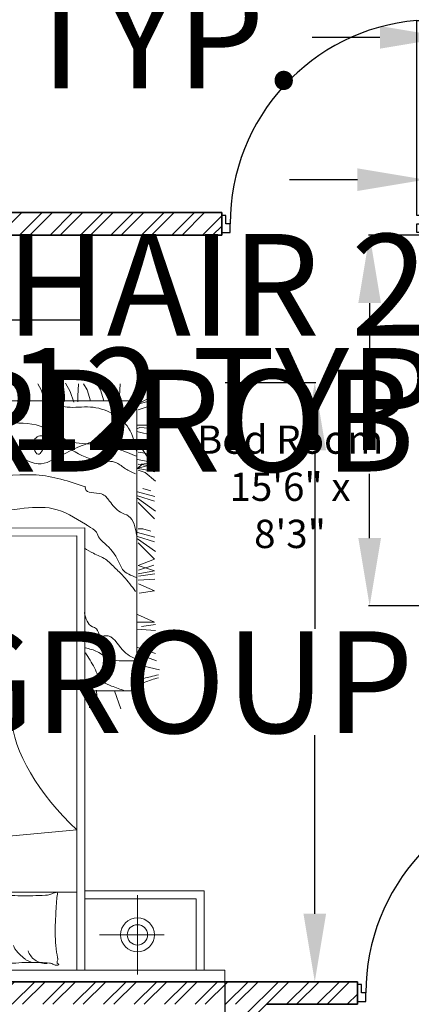
# Model space of a CAD drawing. Units: inches. Extents: x -90 to 536, y -553 to 299.
# Tile 20 of 27: x 137 to 207, y -2 to 173. Entities that reach past the tile are written whole.
import ezdxf

# ---------------------------------------------------------------- set-up
doc = ezdxf.new("R2010")
doc.units = ezdxf.units.IN
for name, color, linetype, lineweight in [('A-ANNO-DIMS', 2, 'Continuous', 18), ('A-AREA-IDEN', 7, 'Continuous', 18), ('A-DOOR', 4, 'Continuous', 25), ('A-FLOR-CASE', 2, 'Continuous', 25), ('A-WALL-PATT', 252, 'Continuous', 13), ('Furniture', 2, 'Continuous', 18), ('Inner Wall', 5, 'Continuous', 35)]:
    doc.layers.add(name, color=color, linetype=linetype, lineweight=lineweight)
doc.styles.get("Standard").update_dxf_attribs({"font": 'arial.ttf'})
doc.dimstyles.get("Standard").update_dxf_attribs({"dimtxt": 18, "dimasz": 12, "dimexe": 0.18, "dimexo": 0.0625, "dimgap": 0.09, "dimtad": 0, "dimtih": 1, "dimtoh": 1, "dimdec": 0, "dimzin": 0, "dimdsep": 46, "dimlunit": 3, "dimtxsty": 'Standard', "dimcen": 0.09, "dimadec": 0, "dimazin": 0, "dimtfac": 1, "dimtdec": 0, "dimtofl": 0, "dimtmove": 0, "dimatfit": 3, "dimfxl": 1, "dimtolj": 1, "dimtzin": 0, "dimarcsym": 0})

# ---------------------------------------------------------------- blocks, each defined once
blk = doc.blocks.new('A$C2B723114')
for p, q in [((0, 2.9047), (2.8274, 2.9047)), ((0, 2.8487), (0, 2.9047)), ((0.4243, 2.8697), (0.4243, 2.4855)), ((2.4742, 2.8697), (2.4742, 2.4855)), ((2.8274, 2.9047), (2.8274, 2.8487)), ((2.8274, 2.8487), (0, 2.8487)), ((0.1012, 2.4649), (0.1012, 2.849)), ((0.1396, 2.5033), (0.1396, 2.849)), ((0.6794, 0.7051), (0.6794, 2.8509)), ((0.7187, 0.7435), (0.7187, 2.8509)), ((2.1776, 2.8509), (2.1776, 0.7454)), ((2.216, 2.8509), (2.216, 0.707)), ((2.6798, 2.5052), (2.6798, 2.8509)), ((2.7182, 2.4668), (2.7182, 2.8509)), ((0.6087, 2.6776), (0.295, 2.6776)), ((2.6586, 2.6776), (2.2821, 2.6776)), ((1.3789, 2.4999), (1.3598, 2.5761)), ((2.0593, 2.4999), (2.0402, 2.5761)), ((0.6766, 2.5033), (0.1396, 2.5033)), ((1.3858, 2.4723), (1.3789, 2.4999)), ((2.0662, 2.4723), (2.0593, 2.4999)), ((2.2188, 2.5052), (2.6798, 2.5052)), ((0.6794, 2.4649), (0.1012, 2.4649)), ((0.7191, 2.47), (2.1778, 2.4719)), ((2.2188, 2.4668), (2.7182, 2.4668)), ((2.1771, 2.3036), (0.718, 2.1685)), ((1.0365, 1.6233), (2.1246, 2.2989)), ((0.5047, 1.5819), (0.5353, 1.4945)), ((0.6174, 1.5819), (0.6232, 1.4916)), ((0.6467, 1.5819), (0.6369, 1.5137)), ((0.6571, 1.4945), (0.6571, 1.5765)), ((2.2287, 1.6076), (2.2523, 1.5035)), ((2.2726, 1.593), (2.3061, 1.5007)), ((2.3067, 1.5881), (2.3373, 1.5007)), ((2.4194, 1.5881), (2.4251, 1.4979)), ((2.4487, 1.5881), (2.4389, 1.5199)), ((2.4591, 1.5007), (2.4591, 1.5828)), ((0.4269, 0.0884), (0.4269, 1.4945)), ((0.4269, 1.4945), (0.6794, 1.4945)), ((2.4685, 1.4964), (2.216, 1.5022)), ((2.4685, 1.4964), (2.4685, 0.0903)), ((0.3172, 1.3923), (0.4213, 1.3687)), ((2.4685, 1.4044), (2.5491, 1.3861)), ((0.3318, 1.3485), (0.4241, 1.3149)), ((2.4596, 1.3659), (2.552, 1.3324)), ((0.3367, 1.3143), (0.4241, 1.2838)), ((2.4645, 1.3318), (2.552, 1.3012)), ((2.4645, 1.2928), (2.5548, 1.2871)), ((2.4645, 1.2635), (2.5328, 1.2733)), ((2.4699, 1.2531), (2.552, 1.2163)), ((2.552, 1.2531), (2.4699, 1.2531)), ((0.3367, 1.2016), (0.427, 1.1959)), ((2.5435, 1.2276), (2.4699, 1.2163)), ((2.4699, 1.2163), (2.5463, 1.1823)), ((0.3367, 1.1724), (0.405, 1.1821)), ((0.4241, 1.162), (0.3421, 1.162)), ((0.3421, 1.162), (0.4241, 1.1252)), ((2.5491, 1.1654), (2.467, 1.1597)), ((2.5463, 1.1455), (2.467, 1.1342)), ((2.5491, 1.1342), (2.4699, 1.1201)), ((2.4699, 1.1201), (2.5491, 1.0946)), ((2.5463, 1.1172), (2.4727, 1.0918)), ((2.5491, 1.0946), (2.4699, 1.0635)), ((2.4699, 1.0635), (2.5491, 0.9842)), ((0.4157, 1.0206), (0.3421, 1.0093)), ((0.3421, 1.0093), (0.4185, 0.9754)), ((2.4642, 1.0267), (2.552, 0.9644)), ((0.4213, 0.9584), (0.3392, 0.9527)), ((2.467, 0.9559), (2.552, 0.9333)), ((2.4699, 0.9785), (2.552, 0.9531)), ((0.4185, 0.9386), (0.3392, 0.9272)), ((0.4213, 0.9272), (0.3421, 0.9131)), ((0.3421, 0.9131), (0.4213, 0.8876)), ((0.4185, 0.9103), (0.3449, 0.8848)), ((2.4642, 0.9389), (2.4869, 0.9276)), ((2.4869, 0.9276), (2.5265, 0.9163)), ((2.5265, 0.9163), (2.5491, 0.9163)), ((0.4213, 0.8876), (0.3421, 0.8565)), ((2.4642, 0.8908), (2.5152, 0.8483)), ((0.3364, 0.8197), (0.4241, 0.7574)), ((0.3421, 0.8565), (0.4213, 0.7772)), ((2.467, 0.8455), (2.5208, 0.8342)), ((2.4699, 0.8172), (2.4925, 0.7974)), ((2.5491, 0.8087), (2.4699, 0.8172)), ((2.5152, 0.8483), (2.5491, 0.837)), ((2.5208, 0.8342), (2.552, 0.8285)), ((2.552, 0.8285), (2.5293, 0.8087)), ((0.3421, 0.7716), (0.4241, 0.7461)), ((2.5491, 0.7606), (2.467, 0.7719)), ((2.4925, 0.7974), (2.535, 0.7889)), ((2.535, 0.7889), (2.552, 0.7861)), ((0.3392, 0.7489), (0.4241, 0.7263)), ((0.359, 0.7206), (0.3987, 0.7093)), ((2.1776, 0.7454), (0.7187, 0.7435)), ((2.4727, 0.7464), (2.467, 0.7408)), ((2.467, 0.7153), (2.5491, 0.7238)), ((2.552, 0.7464), (2.4727, 0.7464)), ((0.3987, 0.7093), (0.4213, 0.7093)), ((2.216, 0.707), (0.6794, 0.7051)), ((0.9938, 0.6115), (1.7555, 0.7064)), ((2.5491, 0.6842), (2.4642, 0.6615)), ((2.552, 0.7096), (2.467, 0.6842)), ((0.3364, 0.6233), (0.4241, 0.561)), ((0.3421, 0.6601), (0.4213, 0.5808)), ((2.5491, 0.6672), (2.4755, 0.6587)), ((2.4755, 0.6474), (2.5548, 0.6276)), ((0.3421, 0.5752), (0.4241, 0.5497)), ((2.4642, 0.6191), (2.4784, 0.6134)), ((2.467, 0.5993), (2.4869, 0.5964)), ((2.4784, 0.6134), (2.5406, 0.6077)), ((2.4869, 0.5964), (2.552, 0.5964)), ((2.5406, 0.6077), (2.552, 0.6134)), ((0.3392, 0.5525), (0.4241, 0.5299)), ((2.467, 0.5313), (2.5491, 0.5596)), ((2.467, 0.5087), (2.5548, 0.5342)), ((2.5548, 0.5342), (2.4699, 0.4889)), ((0.3364, 0.4785), (0.3874, 0.436)), ((0.359, 0.5242), (0.3987, 0.5129)), ((1.4523, 0.5021), (1.1305, 0.4537)), ((0.3392, 0.4332), (0.393, 0.4219)), ((0.3874, 0.436), (0.4213, 0.4247)), ((1.1305, 0.4537), (0.9938, 0.448)), ((0.4213, 0.415), (0.3364, 0.3923)), ((0.4241, 0.2868), (0.3392, 0.415)), ((0.3421, 0.4049), (0.3647, 0.3851)), ((0.4213, 0.3964), (0.3421, 0.4049)), ((0.4213, 0.398), (0.3477, 0.3895)), ((0.3647, 0.3851), (0.4072, 0.3766)), ((0.393, 0.4219), (0.4241, 0.4162)), ((0.4241, 0.4162), (0.4015, 0.3964)), ((2.467, 0.4133), (2.552, 0.4019)), ((2.467, 0.2879), (2.552, 0.4076)), ((0.4213, 0.3377), (0.3392, 0.3491)), ((0.4072, 0.3766), (0.4241, 0.3738)), ((0.3392, 0.2925), (0.4213, 0.3009)), ((0.4241, 0.3236), (0.3449, 0.3236)), ((2.4642, 0.3049), (2.5491, 0.2851)), ((2.467, 0.319), (2.5548, 0.3134)), ((0.3477, 0.2571), (0.427, 0.2373)), ((2.4699, 0.2491), (2.501, 0.2491)), ((2.501, 0.2491), (2.5491, 0.2547)), ((0.3506, 0.2231), (0.4128, 0.2175)), ((0.359, 0.2061), (0.4241, 0.2061)), ((0.4128, 0.2175), (0.4241, 0.2231)), ((2.467, 0.2179), (2.5605, 0.1981)), ((2.467, 0.1981), (2.5491, 0.1613)), ((2.467, 0.184), (2.4982, 0.1755)), ((2.4982, 0.1755), (2.5463, 0.1359)), ((0.3392, 0.1042), (0.4213, 0.1325)), ((0.3392, 0.0815), (0.427, 0.107)), ((0.427, 0.107), (0.3421, 0.0617)), ((1.5674, 0.0962), (1.5844, 0.0453)), ((1.8568, 0.0962), (1.8738, 0.0453)), ((1.9342, 0.0962), (1.9512, 0.0453)), ((2.2236, 0.0962), (2.2406, 0.0453)), ((2.4642, 0.0991), (2.5378, 0.0877)), ((2.4699, 0.1302), (2.535, 0.1104)), ((2.535, 0.1104), (2.5491, 0.0991)), ((2.4685, 0.0903), (0.4269, 0.0884)), ((0.5106, 0.0657), (0.5077, 0.0063)), ((0.5106, 0.094), (0.5106, 0.0657)), ((0.5417, 0.094), (0.5474, 0.0572)), ((0.5474, 0.0572), (0.57, 0.0006)), ((0.587, 0.0884), (0.604, 0.0346)), ((0.6512, 0.0884), (0.6682, 0.0346)), ((0.713, 0.0657), (0.7101, 0.0063)), ((0.713, 0.094), (0.713, 0.0657)), ((0.7334, 0.0943), (0.7503, 0.0434)), ((0.7786, 0.0915), (0.7786, 0.0632)), ((0.7786, 0.0632), (0.7843, 0.0066)), ((0.8739, 0.0884), (0.8908, 0.0346)), ((0.956, 0.0943), (0.973, 0.0434)), ((1.0013, 0.0915), (1.0013, 0.0632)), ((1.0013, 0.0632), (1.007, 0.0066)), ((1.072, 0.0884), (1.089, 0.0346)), ((1.1338, 0.0657), (1.131, 0.0063)), ((1.1338, 0.094), (1.1338, 0.0657)), ((1.1542, 0.0943), (1.1712, 0.0434)), ((1.1995, 0.0915), (1.1995, 0.0632)), ((1.1995, 0.0632), (1.2052, 0.0066)), ((1.4088, 0.0657), (1.406, 0.0063)), ((1.4088, 0.094), (1.4088, 0.0657)), ((1.44, 0.094), (1.4456, 0.0572)), ((1.4456, 0.0572), (1.4683, 0.0006)), ((1.4853, 0.0884), (1.5023, 0.0346)), ((1.6127, 0.0934), (1.6127, 0.0651)), ((1.6127, 0.0651), (1.6184, 0.0085)), ((1.6297, 0.0849), (1.624, 0.0028)), ((1.6693, 0.0623), (1.6608, 0.0028)), ((1.6721, 0.0877), (1.6693, 0.0623)), ((1.7344, 0.0651), (1.7316, 0.0057)), ((1.7344, 0.0934), (1.7344, 0.0651)), ((1.7655, 0.0934), (1.7712, 0.0566)), ((1.7712, 0.0566), (1.7938, 0)), ((1.8108, 0.0877), (1.8278, 0.034)), ((1.9795, 0.0934), (1.9795, 0.0651)), ((1.9795, 0.0651), (1.9852, 0.0085)), ((1.9965, 0.0849), (1.9908, 0.0028)), ((2.0361, 0.0623), (2.0276, 0.0028)), ((2.039, 0.0877), (2.0361, 0.0623)), ((2.1012, 0.0651), (2.0984, 0.0057)), ((2.1012, 0.0934), (2.1012, 0.0651)), ((2.1324, 0.0934), (2.138, 0.0566)), ((2.138, 0.0566), (2.1607, 0)), ((2.1777, 0.0877), (2.1946, 0.034)), ((2.2689, 0.0934), (2.2689, 0.0651)), ((2.2689, 0.0651), (2.2746, 0.0085)), ((2.2859, 0.0849), (2.2802, 0.0028)), ((2.3255, 0.0623), (2.317, 0.0028)), ((2.3284, 0.0877), (2.3255, 0.0623)), ((2.3906, 0.0651), (2.3878, 0.0057)), ((2.3906, 0.0934), (2.3906, 0.0651)), ((2.4218, 0.0934), (2.4274, 0.0566)), ((2.4274, 0.0566), (2.4501, 0)), ((2.467, 0.0877), (2.484, 0.034)), ((2.5378, 0.0877), (2.5463, 0.0821)), ((0.604, 0.0346), (0.621, 0.0063)), ((0.6682, 0.0346), (0.6851, 0.0063)), ((0.7503, 0.0434), (0.773, 0.0037)), ((0.8908, 0.0346), (0.9078, 0.0063)), ((0.973, 0.0434), (0.9957, 0.0037)), ((1.089, 0.0346), (1.106, 0.0063)), ((1.1712, 0.0434), (1.1939, 0.0037)), ((1.5023, 0.0346), (1.5192, 0.0082)), ((1.5844, 0.0453), (1.607, 0.0057)), ((1.8278, 0.034), (1.8448, 0.0057)), ((1.8738, 0.0453), (1.8964, 0.0057)), ((1.9512, 0.0453), (1.9739, 0.0057)), ((2.1946, 0.034), (2.2116, 0.0057)), ((2.2406, 0.0453), (2.2632, 0.0057)), ((2.484, 0.034), (2.501, 0.0057))]:
    blk.add_line(p, q)
for centre, radius in [((0.4243, 2.6776), 0.0821), ((0.4243, 2.6776), 0.0493), ((2.4742, 2.6776), 0.0821), ((2.4742, 2.6776), 0.0493)]:
    blk.add_circle(centre, radius)
for centre, radius, start, end in [((0.8078, 2.821), 0.00214, 160.436, 281.8931), ((0.8088, 2.8207), 0.00315, 111.7883, 160.436), ((0.8162, 2.8021), 0.0232, 94.3025, 111.7883), ((0.8091, 2.8151), 0.00394, 21.9904, 101.8931), ((0.7994, 2.8112), 0.0144, 338.579, 21.9904), ((0.8165, 2.7987), 0.0266, 59.3487, 94.3025), ((0.8554, 2.8643), 0.0497, 239.3487, 264.7408), ((0.8679, 2.7254), 0.0915, 74.0648, 94.2159), ((1.3941, 2.5438), 0.281, 98.4372, 105.744), ((1.3747, 2.6748), 0.1486, 90, 98.4372), ((1.3747, 2.74), 0.0833, 78.7276, 90), ((1.3886, 2.8099), 0.0121, 333.4195, 78.7276), ((1.4882, 2.821), 0.00214, 160.436, 281.8931), ((1.4892, 2.8207), 0.00315, 111.7883, 160.436), ((1.4966, 2.8021), 0.0232, 94.3025, 111.7883), ((1.4895, 2.8151), 0.00394, 21.9904, 101.8931), ((1.4798, 2.8112), 0.0144, 338.579, 21.9904), ((1.4969, 2.7987), 0.0266, 59.3487, 94.3025), ((1.5358, 2.8643), 0.0497, 239.3487, 264.7408), ((1.5483, 2.7254), 0.0915, 74.0648, 94.2159), ((2.0745, 2.5438), 0.281, 98.4372, 105.744), ((2.0551, 2.6748), 0.1486, 90, 98.4372), ((2.0551, 2.74), 0.0833, 78.7276, 90), ((2.069, 2.8099), 0.0121, 333.4195, 78.7276), ((0.8409, 2.7949), 0.0302, 158.579, 188.1335), ((1.0356, 2.8227), 0.2268, 188.1335, 192.1095), ((0.635, 2.7368), 0.1829, 7.6809, 12.1095), ((0.9202, 3.5684), 0.7568, 264.7408, 268.0921), ((0.8679, 2.7254), 0.0915, 53.9136, 74.0648), ((0.9409, 4.189), 1.3777, 268.0921, 270.5757), ((0.8679, 2.7254), 0.0915, 36.1766, 53.9136), ((0.86, 2.6097), 0.2158, 62.7604, 69.1397), ((0.8679, 2.7254), 0.0915, 18.4397, 36.1766), ((0.9466, 3.6164), 0.8051, 270.5757, 274.8018), ((0.9263, 2.7386), 0.0708, 51.6114, 62.7604), ((0.7461, 2.511), 0.3611, 46.1885, 51.6114), ((0.8523, 2.6218), 0.2076, 39.0349, 46.1885), ((1.0364, 2.548), 0.2671, 87.4614, 94.8018), ((1.042, 2.6745), 0.1405, 79.8101, 87.4614), ((1.1532, 3.2931), 0.488, 259.8101, 263.9133), ((1.204, 3.7695), 0.9671, 263.9133, 270), ((1.204, 3.4318), 0.6294, 270, 277.5469), ((1.2573, 3.0292), 0.2233, 277.5469, 285.744), ((1.3713, 2.8186), 0.0315, 274.4002, 333.4195), ((0.923, 2.7382), 0.4535, 0, 6.2324), ((1.5213, 2.7949), 0.0302, 158.579, 188.1335), ((1.716, 2.8227), 0.2268, 188.1335, 192.1095), ((1.3154, 2.7368), 0.1829, 7.6809, 12.1095), ((1.6006, 3.5684), 0.7568, 264.7408, 268.0921), ((1.5483, 2.7254), 0.0915, 53.9136, 74.0648), ((1.6213, 4.189), 1.3777, 268.0921, 270.5757), ((1.5483, 2.7254), 0.0915, 36.1766, 53.9136), ((1.5404, 2.6097), 0.2158, 62.7604, 69.1397), ((1.5483, 2.7254), 0.0915, 18.4397, 36.1766), ((1.627, 3.6164), 0.8051, 270.5757, 274.8018), ((1.6067, 2.7386), 0.0708, 51.6114, 62.7604), ((1.4265, 2.511), 0.3611, 46.1885, 51.6114), ((1.5327, 2.6218), 0.2076, 39.0349, 46.1885), ((1.7168, 2.548), 0.2671, 87.4614, 94.8018), ((1.7224, 2.6745), 0.1405, 79.8101, 87.4614), ((1.8336, 3.2931), 0.488, 259.8101, 263.9133), ((1.8844, 3.7695), 0.9671, 263.9133, 270), ((1.8844, 3.4318), 0.6294, 270, 277.5469), ((1.9377, 3.0292), 0.2233, 277.5469, 285.744), ((2.0517, 2.8186), 0.0315, 274.4002, 333.4195), ((1.6034, 2.7382), 0.4535, 0, 6.2324), ((-0.0181, 2.6487), 0.8418, 3.3687, 7.6809), ((0.9783, 2.7239), 0.0455, 28.3168, 39.0349), ((0.8558, 2.6579), 0.1846, 23.0028, 28.3168), ((1.1884, 2.7382), 0.1881, 350.3156, 0), ((0.6623, 2.6487), 0.8418, 3.3687, 7.6809), ((1.6587, 2.7239), 0.0455, 28.3168, 39.0349), ((1.5362, 2.6579), 0.1846, 23.0028, 28.3168), ((1.8688, 2.7382), 0.1881, 350.3156, 0), ((0.1976, 2.6614), 0.6258, 358.3669, 3.3687), ((0.5722, 2.8434), 0.8132, 347.8016, 350.3156), ((0.878, 2.6614), 0.6258, 358.3669, 3.3687), ((1.2526, 2.8434), 0.8132, 347.8016, 350.3156), ((-0.4351, 2.6794), 1.2587, 356.945, 358.3669), ((1.9648, 2.5659), 0.6074, 171.9949, 177.3351), ((1.6528, 2.6098), 0.2924, 167.8016, 171.9949), ((0.2453, 2.6794), 1.2587, 356.945, 358.3669), ((2.6452, 2.5659), 0.6074, 171.9949, 177.3351), ((2.3332, 2.6098), 0.2924, 167.8016, 171.9949), ((-11.7321, 3.2823), 12.5718, 356.49514, 356.94504), ((1.4204, 2.5912), 0.0624, 177.3351, 194.0452), ((-11.0517, 3.2823), 12.5718, 356.49514, 356.94504), ((2.1008, 2.5912), 0.0624, 177.3351, 194.0452), ((0.5206, 2.5319), 0.2961, 350.0016, 356.4951), ((0.8584, 2.4419), 0.0418, 102.869, 117.2841), ((0.879, 2.3515), 0.1345, 93.574, 102.869), ((0.9376, 1.4146), 1.0732, 90.2865, 93.574), ((0.9586, -2.7845), 5.2724, 89.0296, 90.2865), ((0.9954, -0.6123), 3.0999, 87.3904, 89.0296), ((1.0854, 1.364), 1.1216, 85.3824, 87.3904), ((1.4917, 3.1364), 0.681, 244.6889, 246.5156), ((1.228, 2.691), 0.2121, 267.2509, 281.5586), ((1.4917, 3.1364), 0.681, 246.5156, 248.3423), ((1.4917, 3.1364), 0.681, 248.3423, 250.572), ((1.4917, 3.1364), 0.681, 250.572, 252.8018), ((1.2975, 2.3514), 0.1345, 83.5659, 101.5586), ((1.3002, 2.3754), 0.1104, 72.6136, 83.5659), ((1.201, 2.5319), 0.2961, 350.0016, 356.4951), ((1.5388, 2.4419), 0.0418, 102.869, 117.2841), ((1.5594, 2.3515), 0.1345, 93.574, 102.869), ((1.618, 1.4146), 1.0732, 90.2865, 93.574), ((1.639, -2.7845), 5.2724, 89.0296, 90.2865), ((1.6758, -0.6123), 3.0999, 87.3904, 89.0296), ((1.7658, 1.364), 1.1216, 85.3824, 87.3904), ((2.1721, 3.1364), 0.681, 244.6889, 246.5156), ((1.9084, 2.691), 0.2121, 267.2509, 281.5586), ((2.1721, 3.1364), 0.681, 246.5156, 248.3423), ((2.1721, 3.1364), 0.681, 248.3423, 250.572), ((2.1721, 3.1364), 0.681, 250.572, 252.8018), ((1.9779, 2.3514), 0.1345, 83.5659, 101.5586), ((1.9806, 2.3754), 0.1104, 72.6136, 83.5659), ((0.8298, 2.4774), 0.0178, 170.0016, 196.6978), ((0.8139, 2.4726), 0.00122, 196.6978, 277.1204), ((0.8041, 2.5514), 0.0807, 277.1204, 286.2212), ((0.8068, 2.5419), 0.0707, 286.2212, 297.2841), ((1.28, 3.7729), 1.2952, 265.3824, 267.2509), ((1.3965, 2.6828), 0.2118, 252.6136, 260.5159), ((1.4027, 2.7202), 0.2496, 260.5159, 265.9171), ((1.385, 2.4721), 0.000845, 265.9171, 14.0449), ((1.5102, 2.4774), 0.0178, 170.0016, 196.6978), ((1.4943, 2.4726), 0.00122, 196.6978, 277.1204), ((1.4845, 2.5514), 0.0807, 277.1204, 286.2212), ((1.4872, 2.5419), 0.0707, 286.2212, 297.2841), ((1.9604, 3.7729), 1.2952, 265.3824, 267.2509), ((2.0769, 2.6828), 0.2118, 252.6136, 260.5159), ((2.0831, 2.7202), 0.2496, 260.5159, 265.9171), ((2.0654, 2.4721), 0.000845, 265.9171, 14.0449)]:
    blk.add_arc(centre, radius, start, end)
blk.add_ellipse((0.4962, 1.9132), major_axis=(0.4887, -0.4605), ratio=0.503305, start_param=0.491272, end_param=1.591113)
for points, knots in [([(0.6768, 1.3104), (0.6615, 1.3339), (0.6315, 1.3797), (0.604, 1.4501), (0.5417, 1.4748), (0.5064, 1.4871), (0.4848, 1.4945)], [0, 0, 0, 0, 110.980521, 216.571322, 273.316778, 363.252298, 363.252298, 363.252298, 363.252298]), ([(2.5548, 1.4853), (2.5314, 1.4757), (2.5031, 1.4641), (2.4737, 1.4555), (2.4685, 1.454)], [0, 0, 0, 0, 98.452083, 119.481049, 119.481049, 119.481049, 119.481049]), ([(0.427, 1.4678), (0.4036, 1.4582), (0.3693, 1.4441), (0.3335, 1.4344), (0.3221, 1.4313)], [0, 0, 0, 0, 98.452083, 144.639601, 144.639601, 144.639601, 144.639601]), ([(0.4241, 1.4423), (0.4031, 1.437), (0.3691, 1.4284), (0.3351, 1.4199), (0.3221, 1.4167)], [0, 0, 0, 0, 84.638756, 136.955563, 136.955563, 136.955563, 136.955563]), ([(2.552, 1.4598), (2.5309, 1.4545), (2.5031, 1.4475), (2.4753, 1.4406), (2.4685, 1.4389)], [0, 0, 0, 0, 84.638756, 111.94623, 111.94623, 111.94623, 111.94623]), ([(2.2145, 1.4211), (2.233, 1.4246), (2.2636, 1.4303), (2.2761, 1.3837), (2.3429, 1.3967), (2.3949, 1.3342), (2.4474, 1.3031), (2.4698, 1.2898)], [0, 0, 0, 0, 61.886907, 102.717887, 145.699352, 284.082577, 386.765171, 386.765171, 386.765171, 386.765171]), ([(0.6768, 1.286), (0.6567, 1.2911), (0.6145, 1.3017), (0.5543, 1.3533), (0.4816, 1.349), (0.4362, 1.3493), (0.4233, 1.3493)], [0, 0, 0, 0, 80.250278, 168.388677, 295.908361, 346.663112, 346.663112, 346.663112, 346.663112]), ([(0.4233, 1.3445), (0.4367, 1.3385), (0.464, 1.3264), (0.5129, 1.2848), (0.5456, 1.2161), (0.6131, 1.2349), (0.6142, 1.1913), (0.6642, 1.1806), (0.674, 1.144), (0.6817, 1.1154)], [0, 0, 0, 0, 56.745495, 115.23739, 254.956954, 286.678662, 337.828324, 366.201072, 468.500395, 468.500395, 468.500395, 468.500395]), ([(2.2145, 1.319), (2.2295, 1.319), (2.2678, 1.3192), (2.3288, 1.2705), (2.4143, 1.279), (2.4535, 1.2403), (2.4662, 1.2278)], [0, 0, 0, 0, 57.155505, 146.33427, 287.936209, 355.396728, 355.396728, 355.396728, 355.396728]), ([(2.2182, 1.2059), (2.2419, 1.1958), (2.3116, 1.1659), (2.342, 1.0552), (2.4266, 1.0223), (2.4474, 0.9811), (2.462, 0.9684), (2.4698, 0.9616)], [0, 0, 0, 0, 97.73655, 287.59661, 389.176293, 423.403759, 463.679181, 463.679181, 463.679181, 463.679181]), ([(2.3573, 1.127), (2.3656, 1.1759), (2.3758, 1.2352), (2.3371, 1.1853), (2.3602, 1.1713), (2.3768, 1.1612)], [0, 0, 0, 0, 107.853607, 130.728419, 189.220329, 189.220329, 189.220329, 189.220329]), ([(2.2145, 1.1476), (2.2246, 1.1286), (2.2575, 1.0666), (2.3612, 1.0009), (2.431, 0.9336), (2.4662, 0.8996)], [0, 0, 0, 0, 83.02987, 271.460712, 463.033803, 463.033803, 463.033803, 463.033803]), ([(0.6817, 0.8034), (0.6673, 0.8119), (0.6341, 0.8315), (0.5785, 0.8518), (0.5349, 0.8973), (0.4828, 0.9461), (0.4518, 0.9879), (0.4331, 1.013)], [0, 0, 0, 0, 65.318952, 150.437229, 226.833166, 307.58338, 429.454095, 429.454095, 429.454095, 429.454095]), ([(0.4282, 0.9448), (0.4547, 0.9353), (0.496, 0.9206), (0.5223, 0.8436), (0.5628, 0.7946), (0.6113, 0.7575), (0.6214, 0.7173), (0.6539, 0.7022), (0.672, 0.6897), (0.6768, 0.6864)], [0, 0, 0, 0, 102.299436, 159.044876, 303.717955, 348.579152, 391.138254, 454.581655, 477.456496, 477.456496, 477.456496, 477.456496]), ([(2.2145, 0.823), (2.227, 0.8201), (2.261, 0.8121), (2.261, 0.7401), (2.3352, 0.7659), (2.379, 0.6836), (2.4336, 0.6521), (2.4662, 0.6334)], [0, 0, 0, 0, 46.747668, 127.438174, 179.649794, 280.561838, 429.605131, 429.605131, 429.605131, 429.605131]), ([(0.4282, 0.74), (0.4347, 0.7029), (0.444, 0.6496), (0.5194, 0.6274), (0.555, 0.5807), (0.5975, 0.5243), (0.6789, 0.5415), (0.677, 0.5095), (0.6768, 0.5061)], [0, 0, 0, 0, 130.791737, 187.537266, 286.231946, 353.673191, 460.023761, 472.712403, 472.712403, 472.712403, 472.712403]), ([(2.2218, 0.7246), (2.2595, 0.716), (2.3548, 0.6945), (2.4265, 0.6268), (2.4698, 0.586)], [0, 0, 0, 0, 148.665024, 375.555892, 375.555892, 375.555892, 375.555892]), ([(2.3719, 0.6737), (2.3738, 0.6431), (2.3772, 0.5878), (2.3146, 0.6382), (2.3401, 0.7015), (2.2971, 0.6649), (2.2923, 0.6965), (2.289, 0.7176)], [0, 0, 0, 0, 83.446591, 150.887818, 201.642461, 230.015204, 286.760644, 286.760644, 286.760644, 286.760644]), ([(0.6768, 0.6864), (0.7275, 0.655), (0.8251, 0.5944), (0.9391, 0.606), (0.9938, 0.6115)], [0, 0, 0, 0, 225.995823, 434.686543, 434.686543, 434.686543, 434.686543]), ([(2.2145, 0.5167), (2.1764, 0.5522), (2.1051, 0.6184), (1.9357, 0.5803), (1.9385, 0.6342), (1.9388, 0.6395)], [0, 0, 0, 0, 208.073343, 389.01094, 409.01094, 409.01094, 409.01094, 409.01094]), ([(0.6768, 0.5061), (0.7554, 0.4794), (0.8591, 0.4442), (0.9675, 0.4473), (0.9938, 0.448)], [0, 0, 0, 0, 319.374611, 421.61723, 421.61723, 421.61723, 421.61723]), ([(0.4331, 0.4427), (0.4498, 0.4356), (0.4827, 0.4216), (0.5314, 0.3759), (0.632, 0.3884), (0.6996, 0.3513), (0.7423, 0.3278)], [0, 0, 0, 0, 70.931849, 139.556414, 248.154027, 434.709995, 434.709995, 434.709995, 434.709995]), ([(2.4625, 0.1088), (2.4095, 0.1438), (2.2904, 0.2226), (2.0623, 0.1771), (1.9006, 0.2246), (1.7699, 0.2337), (1.6941, 0.2766), (1.5528, 0.2786), (1.4005, 0.2587), (1.2324, 0.3267), (1.059, 0.2939), (0.9218, 0.426), (0.7359, 0.3204), (0.5586, 0.2391), (0.4502, 0.3116), (0.427, 0.3272)], [0, 0, 0, 0, 239.874704, 538.942419, 850.40885, 893.390315, 1047.998294, 1176.505142, 1437.500972, 1637.333004, 1864.324391, 2089.058767, 2248.736533, 2637.953392, 2744.252142, 2744.252142, 2744.252142, 2744.252142]), ([(1.9771, 0.0962), (1.9286, 0.1117), (1.7864, 0.157), (1.5223, 0.1992), (1.2611, 0.141), (1.0527, 0.2023), (0.8859, 0.1885), (0.76, 0.3042), (0.6211, 0.292), (0.5187, 0.3203), (0.4572, 0.3456), (0.4282, 0.3575)], [0, 0, 0, 0, 198.710624, 582.73994, 1031.873213, 1206.082894, 1423.278209, 1655.952104, 1808.744089, 1945.69963, 2068.229211, 2068.229211, 2068.229211, 2068.229211]), ([(0.8718, 0.2941), (0.8821, 0.3221), (0.9041, 0.3814), (0.9523, 0.2773), (0.8733, 0.2454), (0.8757, 0.2798), (0.8766, 0.2941)], [0, 0, 0, 0, 82.720021, 175.094899, 237.579423, 282.440623, 282.440623, 282.440623, 282.440623]), ([(0.8474, 0.0943), (0.82, 0.1047), (0.757, 0.1287), (0.6201, 0.1029), (0.4623, 0.1837), (0.4372, 0.2936), (0.4282, 0.3331)], [0, 0, 0, 0, 112.422038, 258.341957, 533.791494, 688.286079, 688.286079, 688.286079, 688.286079]), ([(1.2715, 0.221), (1.3344, 0.2172), (1.4529, 0.21), (1.2971, 0.2665), (1.2756, 0.2284), (1.2715, 0.221)], [0, 0, 0, 0, 150.888188, 283.977876, 315.699589, 315.699589, 315.699589, 315.699589])]:
    blk.add_open_spline(points, degree=3, knots=knots)
blk = doc.blocks.new('DOOR-36-A')
for points in [[(35.25, 37.5), (35.25, 3), (34.5, 3), (34.5, 37.5)], [(0, 0), (1.5, 0), (1.5, 1.5), (0.75, 1.5), (0.75, 3), (0, 3)], [(36, 0), (34.5, 0), (34.5, 1.5), (35.25, 1.5), (35.25, 3), (36, 3)]]:
    blk.add_lwpolyline(points, close=True)
blk.add_arc((37.64, 1.5), 36.14, 94.9791, 180)
blk = doc.blocks.new('TV-UNIT')
blk.add_lwpolyline([(15, 65.77), (15, 0), (0, 0), (0, 65.77)], close=True)
blk = doc.blocks.new('*D26')
at = {"layer": 'A-ANNO-DIMS', "color": 0, "lineweight": -2, "transparency": 16777216}
for p, q in [((201.13, 169.45), (189.13, 169.45)), ((213.13, 167), (213.13, 169.63)), ((226.43, 167), (226.43, 169.63)), ((238.43, 169.45), (250.43, 169.45))]:
    blk.add_line(p, q, dxfattribs=at)
at = {"layer": 'A-ANNO-DIMS', "color": 0, "transparency": 16777216}
for points in [[(201.13, 171.45), (201.13, 167.45), (213.13, 169.45)], [(238.43, 171.45), (238.43, 167.45), (226.43, 169.45)]]:
    blk.add_solid(points, dxfattribs=at)
at = {"layer": 'Defpoints', "color": 0, "transparency": 16777216}
for p in [(213.13, 169.45), (213.13, 166.94), (226.43, 166.94)]:
    blk.add_point(p, dxfattribs=at)
at = {"layer": 'A-ANNO-DIMS', "color": 0, "transparency": 16777216, "insert": (146.08, 169.45), "char_height": 18, "attachment_point": 5}
blk.add_mtext('\\A1;13 TYP.', dxfattribs=at)
blk = doc.blocks.new('*D31')
at = {"layer": 'A-ANNO-DIMS', "color": 0, "lineweight": -2, "transparency": 16777216}
for p, q in [((90.45, 119.36), (100.65, 125.67)), ((100.65, 125.67), (112.65, 125.67)), ((78.67, 115.59), (80.34, 112.89)), ((61.33, 104.86), (63, 102.15)), ((52.7, 95.99), (42.5, 89.68))]:
    blk.add_line(p, q, dxfattribs=at)
at = {"layer": 'A-ANNO-DIMS', "color": 0, "transparency": 16777216}
for points in [[(89.4, 121.06), (91.5, 117.65), (80.24, 113.04)], [(51.65, 97.69), (53.76, 94.29), (62.91, 102.31)]]:
    blk.add_solid(points, dxfattribs=at)
at = {"layer": 'Defpoints', "color": 0, "transparency": 16777216}
for p in [(78.63, 115.64), (80.24, 113.04), (61.3, 104.91)]:
    blk.add_point(p, dxfattribs=at)
at = {"layer": 'A-ANNO-DIMS', "color": 0, "transparency": 16777216, "insert": (199.06, 125.67), "char_height": 18, "attachment_point": 5}
blk.add_mtext('\\A1;CHAIR 20 TYP.', dxfattribs=at)
blk = doc.blocks.new('*D33')
at = {"layer": 'A-ANNO-DIMS', "color": 0, "lineweight": -2, "transparency": 16777216}
for p, q in [((173.76, 108.4), (189.77, 108.4)), ((189.59, 96.4), (189.59, 64.83)), ((189.59, 14.45), (189.59, 46.02)), ((173.76, 2.45), (189.77, 2.45))]:
    blk.add_line(p, q, dxfattribs=at)
at = {"layer": 'A-ANNO-DIMS', "color": 0, "transparency": 16777216}
for points in [[(187.59, 96.4), (191.59, 96.4), (189.59, 108.4)], [(187.59, 14.45), (191.59, 14.45), (189.59, 2.45)]]:
    blk.add_solid(points, dxfattribs=at)
at = {"layer": 'Defpoints', "color": 0, "transparency": 16777216}
for p in [(173.7, 108.4), (173.7, 2.45), (189.59, 2.45)]:
    blk.add_point(p, dxfattribs=at)
at = {"layer": 'A-ANNO-DIMS', "color": 0, "transparency": 16777216, "insert": (189.59, 55.42), "char_height": 18, "attachment_point": 5}
blk.add_mtext('\\A1;BED GROUP 106 TYP.', dxfattribs=at)
blk = doc.blocks.new('*D34')
at = {"layer": 'A-ANNO-DIMS', "color": 0, "lineweight": -2, "transparency": 16777216}
for p, q in [((70.57, 2.38), (70.57, -13.63)), ((173.7, 2.38), (173.7, -13.63)), ((58.57, -13.45), (46.57, -13.45)), ((185.7, -13.45), (197.7, -13.45))]:
    blk.add_line(p, q, dxfattribs=at)
at = {"layer": 'A-ANNO-DIMS', "color": 0, "transparency": 16777216}
for points in [[(58.57, -11.45), (58.57, -15.45), (70.57, -13.45)], [(185.7, -11.45), (185.7, -15.45), (173.7, -13.45)]]:
    blk.add_solid(points, dxfattribs=at)
at = {"layer": 'Defpoints', "color": 0, "transparency": 16777216}
for p in [(70.57, 2.45), (173.7, 2.45), (70.57, -13.45)]:
    blk.add_point(p, dxfattribs=at)
at = {"layer": 'A-ANNO-DIMS', "color": 0, "transparency": 16777216, "insert": (122.13, -13.45), "char_height": 18, "attachment_point": 5}
blk.add_mtext('\\A1;103 TYP.', dxfattribs=at)
blk = doc.blocks.new('*D37')
at = {"layer": 'A-ANNO-DIMS', "color": 0, "lineweight": -2, "transparency": 16777216}
for p, q in [((23.09, 105.5), (11.09, 105.5)), ((35.09, 103.75), (35.09, 105.68)), ((47.13, 103.75), (47.13, 105.68)), ((59.13, 105.5), (71.13, 105.5))]:
    blk.add_line(p, q, dxfattribs=at)
at = {"layer": 'A-ANNO-DIMS', "color": 0, "transparency": 16777216}
for points in [[(23.09, 107.5), (23.09, 103.5), (35.09, 105.5)], [(59.13, 107.5), (59.13, 103.5), (47.13, 105.5)]]:
    blk.add_solid(points, dxfattribs=at)
at = {"layer": 'Defpoints', "color": 0, "transparency": 16777216}
for p in [(47.13, 105.5), (35.09, 103.69), (47.13, 103.69)]:
    blk.add_point(p, dxfattribs=at)
at = {"layer": 'A-ANNO-DIMS', "color": 0, "transparency": 16777216, "insert": (147.42, 105.5), "char_height": 18, "attachment_point": 5}
blk.add_mtext('\\A1;PIER 12 TYP.', dxfattribs=at)
blk = doc.blocks.new('*D39')
at = {"layer": 'A-ANNO-DIMS', "color": 0, "lineweight": -2, "transparency": 16777216}
for p, q in [((209.07, 134.45), (199.12, 134.45)), ((199.3, 122.45), (199.3, 111.07)), ((199.3, 80.89), (199.3, 92.26)), ((209.07, 68.89), (199.12, 68.89))]:
    blk.add_line(p, q, dxfattribs=at)
at = {"layer": 'A-ANNO-DIMS', "color": 0, "transparency": 16777216}
for points in [[(197.3, 122.45), (201.3, 122.45), (199.3, 134.45)], [(197.3, 80.89), (201.3, 80.89), (199.3, 68.89)]]:
    blk.add_solid(points, dxfattribs=at)
at = {"layer": 'Defpoints', "color": 0, "transparency": 16777216}
for p in [(199.3, 134.45), (209.13, 134.45), (209.13, 68.89)]:
    blk.add_point(p, dxfattribs=at)
at = {"layer": 'A-ANNO-DIMS', "color": 0, "transparency": 16777216, "insert": (199.3, 101.67), "char_height": 18, "attachment_point": 5}
blk.add_mtext('\\A1;WARDROBE 66 TYP.', dxfattribs=at)
blk = doc.blocks.new('*D40')
at = {"layer": 'A-ANNO-DIMS', "color": 0, "lineweight": -2, "transparency": 16777216}
for p, q in [((197.13, 144.28), (185.13, 144.28)), ((209.13, 134.51), (209.13, 144.46)), ((233.13, 134.51), (233.13, 144.46)), ((245.13, 144.28), (257.13, 144.28))]:
    blk.add_line(p, q, dxfattribs=at)
at = {"layer": 'A-ANNO-DIMS', "color": 0, "transparency": 16777216}
for points in [[(197.13, 146.28), (197.13, 142.28), (209.13, 144.28)], [(245.13, 146.28), (245.13, 142.28), (233.13, 144.28)]]:
    blk.add_solid(points, dxfattribs=at)
at = {"layer": 'Defpoints', "color": 0, "transparency": 16777216}
for p in [(233.13, 144.28), (209.13, 134.45), (233.13, 134.45)]:
    blk.add_point(p, dxfattribs=at)
at = {"layer": 'A-ANNO-DIMS', "color": 0, "transparency": 16777216, "insert": (301.18, 144.28), "char_height": 18, "attachment_point": 5}
blk.add_mtext('\\A1;24 TYP.', dxfattribs=at)
blk = doc.blocks.new('*D53')
at = {"layer": 'A-ANNO-DIMS', "color": 0, "lineweight": -2, "transparency": 16777216}
for p, q in [((35.09, 103.75), (35.09, 287.38)), ((407.13, -63.49), (407.13, 287.38)), ((47.09, 287.2), (183.7, 287.2)), ((395.13, 287.2), (258.52, 287.2))]:
    blk.add_line(p, q, dxfattribs=at)
at = {"layer": 'A-ANNO-DIMS', "color": 0, "transparency": 16777216}
for points in [[(47.09, 289.2), (47.09, 285.2), (35.09, 287.2)], [(395.13, 289.2), (395.13, 285.2), (407.13, 287.2)]]:
    blk.add_solid(points, dxfattribs=at)
at = {"layer": 'Defpoints', "color": 0, "transparency": 16777216}
for p in [(407.13, 287.2), (35.09, 103.69), (407.13, -63.55)]:
    blk.add_point(p, dxfattribs=at)
at = {"layer": 'A-ANNO-DIMS', "color": 0, "transparency": 16777216, "insert": (221.11, 287.2), "char_height": 18, "attachment_point": 5}
blk.add_mtext('\\A1;372.04', dxfattribs=at)

msp = doc.modelspace()

# ---------------------------------------------------------------- hatches: boundary and pattern name
at = {"layer": 'A-WALL-PATT'}
h = msp.add_hatch(dxfattribs=at)
h.set_pattern_fill('ANSI32', color=256, scale=0.4)
h.set_pattern_definition([(45, (-88.8105, -603.6155), (-2.694077, 2.694077), []), (45, (-87.0145, -603.6155), (-2.694077, 2.694077), [])])
h.paths.add_polyline_path([(285.1317, 246.4462), (131.1317, 246.4462), (131.1317, 237.4462), (285.1317, 237.4462)])
h.paths.add_polyline_path([(122.1317, 237.4462), (113.1317, 237.4462), (113.1317, 152.4462), (122.1317, 152.4462), (122.1317, 166.4704)])
h.paths.add_polyline_path([(303.1317, 237.4462), (294.1317, 237.4462), (294.1317, 152.4462), (303.1317, 152.4462)])
h.paths.add_polyline_path([(47.1317, 91.9277), (38.1317, 91.9277), (38.1317, -6.5538), (77.1317, -6.5538), (77.1317, 2.4462), (70.5655, 2.4462), (47.1317, 2.4462)])
h.paths.add_polyline_path([(83.052, -61.5538), (47.1317, -61.5538), (47.1317, -24.5538), (38.1317, -24.5538), (38.1317, -70.5538), (74.052, -70.5538), (74.052, -223.5538), (38.1317, -223.5538), (38.1317, -503.5538), (92.1317, -503.5538), (92.1317, -437.5538), (191.1317, -437.5538), (191.1317, -428.5538), (83.1317, -428.5538), (83.1317, -494.5538), (47.1317, -494.5538), (47.1317, -232.5538), (83.052, -232.5538), (83.052, -70.5538)])
h.paths.add_polyline_path([(407.1317, -63.5538), (381.1317, -63.5538), (381.1317, 91.9277), (372.1317, 91.9277), (372.1317, 32.8805), (372.1317, -63.5538), (306.5745, -63.5538), (237.1317, -63.5538), (237.1317, -38.5538), (233.1317, -38.5538), (233.1317, -71.5538), (398.1317, -71.5538), (398.1317, -152.5538), (233.1317, -152.5538), (233.1317, -161.5538), (398.1317, -161.5538), (398.1317, -368.5538), (233.1317, -368.5538), (233.1317, -377.5538), (407.1317, -377.5538), (407.1317, -161.5538)])
h.paths.add_polyline_path([(261.1317, -422.5538), (252.1317, -422.5538), (252.1317, -428.5538), (233.1317, -428.5538), (233.1317, -437.5538), (261.1317, -437.5538)])
h.paths.add_polyline_path([(191.1317, -368.5538), (180.1317, -368.5538), (180.1317, -335.5538), (131.5919, -335.5538), (131.5919, -344.5538), (171.1317, -344.5538), (171.1317, -392.5538), (180.1317, -392.5538), (180.1317, -377.5538), (191.1317, -377.5538)], flags=17)
h.paths.add_polyline_path([(180.1317, -223.5538), (152.1317, -223.5538), (152.1317, -227.5538), (176.1317, -227.5538), (176.1317, -335.5538), (180.1317, -335.5538)], flags=17)
h.paths.add_polyline_path([(131.5919, -335.5538), (83.1317, -335.5538), (83.1317, -339.5538), (83.1317, -392.5538), (87.1317, -392.5538), (87.1317, -339.5538), (131.5919, -339.5538)], flags=17)
h.paths.add_polyline_path([(197.1317, 2.4462), (77.1317, 2.4462), (77.1317, -1.5538), (113.1317, -1.5538), (113.1317, -71.5538), (181.1317, -71.5538), (181.1317, -67.5538), (117.1317, -67.5538), (117.1317, -1.5538), (177.1317, -1.5538), (177.1317, -37.5538), (181.1317, -37.5538), (181.1317, -1.5538), (197.1317, -1.5538)])
h.paths.add_polyline_path([(173.1317, 138.4462), (122.1317, 138.4462), (122.1317, 134.4462), (173.1317, 134.4462)])
h.paths.add_polyline_path([(213.1317, 237.4462), (209.1317, 237.4462), (209.1317, 134.4462), (233.1317, 134.4462), (233.1317, 68.8889), (233.1317, -2.5538), (237.1317, -2.5538), (237.1317, 134.4462), (258.1317, 134.4462), (258.1317, 138.4462), (213.1317, 138.4462)])

# ---------------------------------------------------------------- linework, layer by layer
at = {"layer": 'Inner Wall'}
for p, q in [((173.1317, 138.4462), (122.1317, 138.4462)), ((173.1317, 138.4462), (173.1317, 134.4462)), ((173.1317, 134.4462), (122.1317, 134.4462)), ((197.1317, 2.4462), (47.1317, 2.4462)), ((197.1317, 2.4462), (197.1317, -1.5538)), ((197.1317, -1.5538), (181.1317, -1.5538))]:
    msp.add_line(p, q, dxfattribs=at)

# ---------------------------------------------------------------- block references
at = {"layer": 'A-DOOR'}
for p in [(173.1317, 134.9462), (197.1317, -1.0538)]:
    msp.add_blockref('DOOR-36-A', p, dxfattribs=at)
at = {"layer": 'A-FLOR-CASE', "rotation": 90.00000000000007}
msp.add_blockref('TV-UNIT', (149.0162, 119.4462), dxfattribs=at)
at = {"layer": 'Furniture', "xscale": 36.47664764473289, "yscale": 36.47664764473289, "zscale": 36.47664764473289, "rotation": 180}
msp.add_blockref('A$C2B723114', (173.698, 108.4009), dxfattribs=at)

# ---------------------------------------------------------------- texts
at = {"layer": 'A-AREA-IDEN', "insert": (202.8337, 100.8066), "char_height": 5, "attachment_point": 3}
msp.add_mtext_dynamic_manual_height_columns('\\pxqc;{\\fTimes New Roman|b0|i0|c0|p18;Bed Room\\P15\'6" x 8\'3"}', width=35.23368, gutter_width=12.5, heights=[0], dxfattribs=at)

# ---------------------------------------------------------------- dimensions: what is measured, and where the dimension line sits
at = {"layer": 'A-ANNO-DIMS'}
dim = msp.add_linear_dim(base=(407.1317, 287.2012), p1=(35.0873, 103.6916), p2=(407.1317, -63.5538), dimstyle='Standard', override={"dimdec": 2, "dimlfac": 1, "dimrnd": 0, "dimzin": 0, "dimdsep": 46, "dimlunit": 2}, dxfattribs=at)
dim.commit()
dim.dimension.update_dxf_attribs({"geometry": '*D53', "text_midpoint": (221.1095, 287.2012)})
for base, p1, p2, angle, text, picture, middle in [((213.1317, 169.4531), (226.4312, 166.9352), (213.1317, 166.9352), 180, '<> TYP.', '*D26', (146.0799, 169.4531)), ((80.2442, 113.0397), (61.2964, 104.9085), (78.6344, 115.6404), 31.756702, 'CHAIR <> TYP.', '*D31', (199.0577, 125.6712)), ((199.2981, 134.4462), (209.1317, 68.8889), (209.1317, 134.4462), 90, 'WARDROBE <> TYP.', '*D39', (199.2981, 101.6676)), ((189.5912, 2.4462), (173.698, 108.4009), (173.698, 2.4462), 270, 'BED GROUP <> TYP.', '*D33', (189.5912, 55.4235)), ((70.5655, -13.447), (173.698, 2.4462), (70.5655, 2.4462), 180, '<> TYP.', '*D34', (122.1317, -13.447))]:
    dim = msp.add_linear_dim(base=base, p1=p1, p2=p2, angle=angle, text=text, dimstyle='Standard', override={"dimdec": 0, "dimlfac": 1, "dimrnd": 0, "dimzin": 0, "dimdsep": 46, "dimlunit": 2}, dxfattribs=at)
    dim.commit()
    dim.dimension.update_dxf_attribs({"geometry": picture, "text_midpoint": middle})
for base, p1, p2, text, picture, middle in [((233.1317, 144.2798), (209.1317, 134.4462), (233.1317, 134.4462), '<> TYP.', '*D40', (301.1842, 144.2798)), ((47.1317, 105.4983), (35.0873, 103.6916), (47.1317, 103.6916), 'PIER <> TYP.', '*D37', (147.4209, 105.4983))]:
    dim = msp.add_linear_dim(base=base, p1=p1, p2=p2, text=text, dimstyle='Standard', override={"dimdec": 0, "dimlfac": 1, "dimrnd": 0, "dimzin": 0, "dimdsep": 46, "dimlunit": 2}, dxfattribs=at)
    dim.commit()
    dim.dimension.update_dxf_attribs({"geometry": picture, "text_midpoint": middle})

doc.saveas('drawing.dxf')
